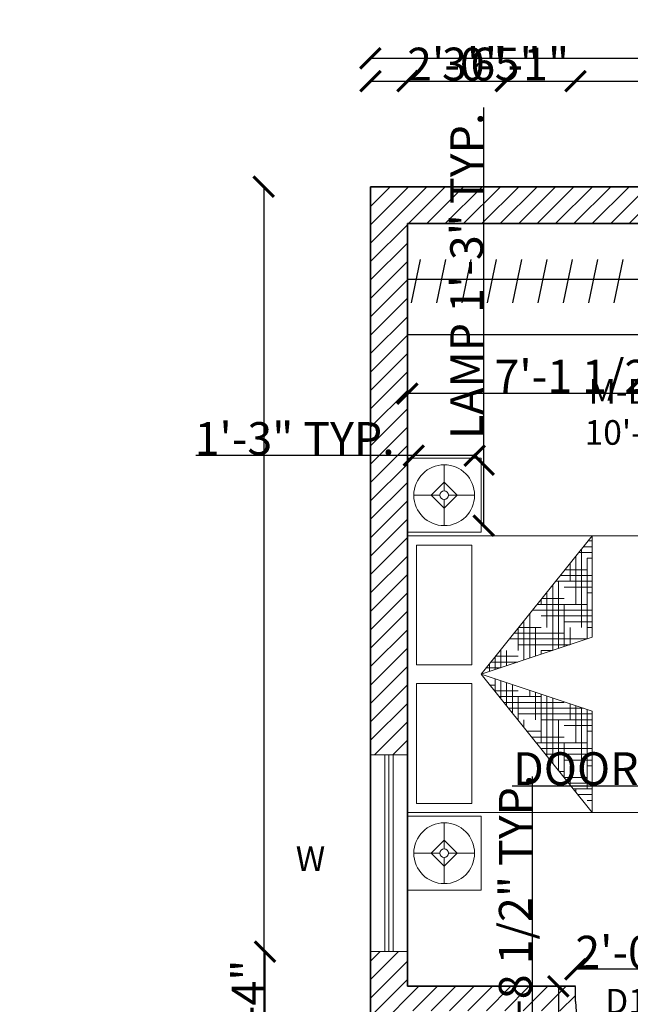
# Model space of a CAD drawing. Units: inches. Extents: x 2094 to 2639, y 1426 to 1997.
# Tile 5 of 8: x 2094 to 2243, y 1730 to 1970. Entities that reach past the tile are written whole.
import ezdxf

# ---------------------------------------------------------------- set-up
doc = ezdxf.new("R2010")
doc.units = ezdxf.units.IN
for name, color, linetype, lineweight in [('A-ANNO-DIMS', 2, 'Continuous', 18), ('A-ANNO-TEXT', 7, 'Continuous', 18), ('A-AREA-IDEN', 7, 'Continuous', 25), ('A-FLOR-CASE', 8, 'Continuous', 25), ('A-FURN', 8, 'Continuous', 18), ('A-WALL-PATT', 8, 'Continuous', 13), ('Doors', 34, 'Continuous', 25), ('Walls', 7, 'Continuous', 35), ('Windows', 150, 'Continuous', 18)]:
    doc.layers.add(name, color=color, linetype=linetype, lineweight=lineweight)
doc.styles.get("Standard").update_dxf_attribs({"font": 'arial.ttf'})
doc.dimstyles.get("Standard").update_dxf_attribs({"dimtxt": 8, "dimasz": 5, "dimexe": 0.18, "dimexo": 0.0625, "dimgap": 0.09, "dimtad": 1, "dimdec": 1, "dimzin": 0, "dimdsep": 46, "dimlunit": 4, "dimtxsty": 'Standard', "dimblk": 'ARCHTICK', "dimcen": 0.09, "dimse1": 1, "dimse2": 1, "dimadec": 0, "dimazin": 0, "dimtfac": 1, "dimtdec": 1, "dimtofl": 0, "dimtmove": 0, "dimatfit": 3, "dimfxl": 1, "dimtolj": 1, "dimtzin": 0, "dimarcsym": 0})

# ---------------------------------------------------------------- blocks, each defined once
blk = doc.blocks.new('*X3')
at = {"color": 0}
for p, q in [((20.199, 14.7812), (20.2772, 14.7812)), ((20.25, 14.8125), (20.2772, 14.8125)), ((20.1562, 14.625), (20.1562, 14.7281)), ((20.1739, 14.75), (20.2772, 14.75)), ((20.1875, 14.75), (20.1875, 14.7669)), ((20.25, 14.3194), (20.25, 14.75)), ((20.1236, 14.6875), (20.25, 14.6875)), ((20.125, 14.5), (20.125, 14.6893)), ((20.1487, 14.7188), (20.2772, 14.7188)), ((20.0938, 14.375), (20.0938, 14.6504)), ((20.0984, 14.6562), (20.125, 14.6562)), ((20.2188, 14.3091), (20.2188, 14.625)), ((20.25, 14.625), (20.2772, 14.625)), ((20.0312, 14.2469), (20.0312, 14.5727)), ((20.0625, 14.2573), (20.0625, 14.6116)), ((20.125, 14.5938), (20.2772, 14.5938)), ((19.9979, 14.5312), (20.2772, 14.5312)), ((20.023, 14.5625), (20.2772, 14.5625)), ((19.9476, 14.4688), (20.125, 14.4688)), ((19.9727, 14.5), (20.25, 14.5)), ((20, 14.2366), (20, 14.5)), ((20.1875, 14.2987), (20.1875, 14.5)), ((19.9062, 14.375), (19.9062, 14.4174)), ((19.9225, 14.4375), (20, 14.4375)), ((20.25, 14.4375), (20.2772, 14.4375)), ((19.875, 14.25), (19.875, 14.3785)), ((19.9688, 14.2262), (19.9688, 14.375)), ((20, 14.375), (20.2772, 14.375)), ((20.125, 14.4062), (20.2772, 14.4062)), ((20.1562, 14.2884), (20.1562, 14.375)), ((19.8125, 14.1744), (19.8125, 14.3008)), ((19.8219, 14.3125), (20.2291, 14.3125)), ((19.8438, 14.1848), (19.8438, 14.3397)), ((19.875, 14.3438), (20.2772, 14.3438)), ((19.7716, 14.25), (20, 14.25)), ((19.7812, 14.1641), (19.7812, 14.262)), ((19.7967, 14.2812), (20.125, 14.2812)), ((19.9375, 14.2159), (19.9375, 14.25)), ((19.7465, 14.2188), (19.875, 14.2188)), ((19.75, 14.1537), (19.75, 14.2231)), ((19.7213, 14.1875), (19.75, 14.1875)), ((19.7018, 14.0938), (19.7786, 14.0938)), ((19.7188, 14.0726), (19.7188, 14.1136)), ((19.75, 14.0338), (19.75, 14.1032)), ((19.7812, 13.9949), (19.7812, 14.0929)), ((19.7269, 14.0625), (19.8728, 14.0625)), ((19.8125, 14), (19.8125, 14.0825)), ((19.9062, 13.8396), (19.9062, 14.0514)), ((19.9375, 13.8007), (19.9375, 14.0411)), ((19.752, 14.0312), (19.875, 14.0312)), ((19.875, 13.8784), (19.875, 14)), ((19.9688, 13.875), (19.9688, 14.0307)), ((20, 14), (20, 14.0204)), ((20, 14), (20.0614, 14)), ((20.0625, 13.6454), (20.0625, 13.9996)), ((20.0938, 13.625), (20.0938, 13.9893)), ((19.8275, 13.9375), (20.25, 13.9375)), ((19.875, 13.9688), (20.1557, 13.9688)), ((20.125, 13.75), (20.125, 13.9789)), ((20.1562, 13.875), (20.1562, 13.9686)), ((20.25, 13.5), (20.25, 13.9375)), ((19.8526, 13.9062), (20.125, 13.9062)), ((19.8777, 13.875), (20, 13.875)), ((20.0312, 13.6842), (20.0312, 13.875)), ((20.2188, 13.4511), (20.2188, 13.875)), ((20.25, 13.875), (20.2772, 13.875)), ((20.125, 13.8438), (20.2772, 13.8438)), ((19.9532, 13.7812), (20.2772, 13.7812)), ((20, 13.8125), (20.2772, 13.8125)), ((19.9783, 13.75), (20.25, 13.75)), ((20, 13.723), (20, 13.75)), ((20.0035, 13.7188), (20.125, 13.7188)), ((20.1875, 13.49), (20.1875, 13.75)), ((20.25, 13.6875), (20.2772, 13.6875)), ((20.0789, 13.625), (20.2772, 13.625)), ((20.125, 13.6562), (20.2772, 13.6562)), ((20.1562, 13.5288), (20.1562, 13.625)), ((20.104, 13.5938), (20.2772, 13.5938)), ((20.1292, 13.5625), (20.25, 13.5625)), ((20.25, 13.5), (20.2772, 13.5)), ((20.2046, 13.4688), (20.2772, 13.4688)), ((20.2297, 13.4375), (20.2772, 13.4375)), ((20.2549, 13.4062), (20.2772, 13.4062))]:
    blk.add_line(p, q, dxfattribs=at)
blk = doc.blocks.new('MAT-P13')
for p, q in [((-1.17, 0), (-1.17, -0.4)), ((-1.17, 0), (-0.77, 0)), ((-0.77, 0), (-0.77, -0.4)), ((-0.75, 0), (0.75, 0)), ((-0.75, 0), (-0.75, -1.9)), ((0.75, 0), (0.75, -1.9)), ((0.77, 0), (1.17, 0)), ((0.77, 0), (0.77, -0.4)), ((1.17, 0), (1.17, -0.4)), ((-0.7, -0.05), (-0.7, -0.35)), ((-0.7, -0.05), (-0.05, -0.05)), ((-0.05, -0.35), (-0.05, -0.05)), ((0.05, -0.05), (0.7, -0.05)), ((0.05, -0.35), (0.05, -0.05)), ((0.7, -0.05), (0.7, -0.35)), ((-0.7, -0.35), (-0.05, -0.35)), ((0.05, -0.35), (0.7, -0.35)), ((-1.17, -0.4), (-0.77, -0.4)), ((-0.75, -1.0034), (0, -0.4)), ((0, -0.4), (-0.75, -1.0034)), ((0, -0.4), (-0.2, -1.0034)), ((0, -0.4), (0.2, -1.0034)), ((0, -0.4), (0.75, -1.0034)), ((0.77, -0.4), (1.17, -0.4)), ((-0.75, -1.0034), (-0.2, -1.0034)), ((0.2, -1.0034), (0.75, -1.0034)), ((0.75, -1.9), (-0.75, -1.9))]:
    blk.add_line(p, q)
at = {"xscale": -1, "rotation": 90}
blk.add_blockref('*X3', (14.1285, 19.2738), dxfattribs=at)
blk = doc.blocks.new('Lamp - Table')
for p, q in [((0, 7), (0, 1)), ((0, 3), (-3, 0)), ((3, 0), (0, 3)), ((-1, 0), (-7, 0)), ((-3, 0), (0, -3)), ((0, -3), (3, 0)), ((1, 0), (7, 0)), ((0, -1), (0, -7))]:
    blk.add_line(p, q)
for radius in [7, 1]:
    blk.add_circle((0, 0), radius)
blk = doc.blocks.new('AP0B05')
for p, q in [((35, 100), (35, 880)), ((75, 100), (75, 878.9)), ((35, 100), (35, -20)), ((815, 100), (815, -20))]:
    blk.add_line(p, q)
blk.add_lwpolyline([(35, 100), (75, 100)])
blk.add_arc((-2.4, 62.6), 818.3, 2.62122, 87.37878)
blk = doc.blocks.new('_ArchTick')
at = {"color": 0, "linetype": 'ByBlock', "const_width": 0.15}
blk.add_lwpolyline([(-0.5, -0.5), (0.5, 0.5)], dxfattribs=at)
blk = doc.blocks.new('*D13')
at = {"layer": 'A-ANNO-DIMS', "color": 0, "lineweight": -2, "transparency": 16777216}
blk.add_line((2180.06, 1960.22), (2537.06, 1960.22), dxfattribs=at)
at = {"layer": 'Defpoints', "color": 0, "transparency": 16777216}
for p in [(2537.06, 1960.22), (2180.06, 1928.9), (2537.06, 1928.9)]:
    blk.add_point(p, dxfattribs=at)
at = {"layer": 'A-ANNO-DIMS', "color": 0, "lineweight": -2, "transparency": 16777216, "xscale": 5, "yscale": 5, "zscale": 5, "rotation": 180}
blk.add_blockref('_ArchTick', (2180.06, 1960.22), dxfattribs=at)
at = {"layer": 'A-ANNO-DIMS', "color": 0, "lineweight": -2, "transparency": 16777216, "xscale": 5, "yscale": 5, "zscale": 5}
blk.add_blockref('_ArchTick', (2537.06, 1960.22), dxfattribs=at)
at = {"layer": 'A-ANNO-DIMS', "color": 0, "transparency": 16777216, "insert": (2358.56, 1964.39), "char_height": 8, "attachment_point": 5}
blk.add_mtext('\\A1;29\'-9"', dxfattribs=at)
blk = doc.blocks.new('*D14')
at = {"layer": 'A-ANNO-DIMS', "color": 0, "lineweight": -2, "transparency": 16777216}
blk.add_line((2154, 1928.9), (2154, 1459.9), dxfattribs=at)
at = {"layer": 'Defpoints', "color": 0, "transparency": 16777216}
for p in [(2180.06, 1928.9), (2154, 1459.9), (2180.06, 1459.9)]:
    blk.add_point(p, dxfattribs=at)
at = {"layer": 'A-ANNO-DIMS', "color": 0, "lineweight": -2, "transparency": 16777216, "xscale": 5, "yscale": 5, "zscale": 5}
for p, rotation in [((2154, 1928.9), 90), ((2154, 1459.9), 270)]:
    blk.add_blockref('_ArchTick', p, dxfattribs=dict(at, rotation=rotation))
at = {"layer": 'A-ANNO-DIMS', "color": 0, "transparency": 16777216, "insert": (2149.82, 1694.4), "char_height": 8, "attachment_point": 5, "rotation": 90}
blk.add_mtext('\\A1;39\'-1"', dxfattribs=at)
blk = doc.blocks.new('WIN-48IN')
for p, q in [((0, 5.5), (48, 5.5)), ((0, 4.5), (48, 4.5)), ((0, 3.5), (48, 3.5))]:
    blk.add_line(p, q)
blk.add_lwpolyline([(0, 0), (48, 0), (48, 9), (0, 9)], close=True)
blk = doc.blocks.new('*D23')
at = {"layer": 'A-ANNO-DIMS', "color": 0, "lineweight": -2, "transparency": 16777216}
for p, q in [((2225.93, 1733.9), (2225.93, 1706.16)), ((2225.93, 1706.16), (2225.93, 1624.84))]:
    blk.add_line(p, q, dxfattribs=at)
at = {"layer": 'Defpoints', "color": 0, "transparency": 16777216}
for p in [(2230.09, 1733.9), (2225.93, 1706.16), (2230.09, 1706.16)]:
    blk.add_point(p, dxfattribs=at)
at = {"layer": 'A-ANNO-DIMS', "color": 0, "lineweight": -2, "transparency": 16777216, "xscale": 5, "yscale": 5, "zscale": 5}
for p, rotation in [((2225.93, 1733.9), 90), ((2225.93, 1706.16), 270)]:
    blk.add_blockref('_ArchTick', p, dxfattribs=dict(at, rotation=rotation))
at = {"layer": 'A-ANNO-DIMS', "color": 0, "transparency": 16777216, "insert": (2221.69, 1663), "char_height": 8, "attachment_point": 5, "rotation": 90}
blk.add_mtext('\\A1;DOOR 2\'-3 1/2"', dxfattribs=at)
blk = doc.blocks.new('*D24')
at = {"layer": 'A-ANNO-DIMS', "color": 0, "lineweight": -2, "transparency": 16777216}
blk.add_line((2254.12, 1738.06), (2230.09, 1738.06), dxfattribs=at)
at = {"layer": 'Defpoints', "color": 0, "transparency": 16777216}
for p in [(2230.09, 1738.06), (2230.09, 1733.9), (2254.12, 1733.9)]:
    blk.add_point(p, dxfattribs=at)
at = {"layer": 'A-ANNO-DIMS', "color": 0, "lineweight": -2, "transparency": 16777216, "xscale": 5, "yscale": 5, "zscale": 5, "rotation": 180}
blk.add_blockref('_ArchTick', (2230.09, 1738.06), dxfattribs=at)
at = {"layer": 'A-ANNO-DIMS', "color": 0, "lineweight": -2, "transparency": 16777216, "xscale": 5, "yscale": 5, "zscale": 5}
blk.add_blockref('_ArchTick', (2254.12, 1738.06), dxfattribs=at)
at = {"layer": 'A-ANNO-DIMS', "color": 0, "transparency": 16777216, "insert": (2242.11, 1742.23), "char_height": 8, "attachment_point": 5}
blk.add_mtext('\\A1;2\'-0"', dxfattribs=at)
blk = doc.blocks.new('*D25')
at = {"layer": 'A-ANNO-DIMS', "color": 0, "lineweight": -2, "transparency": 16777216}
for p, q in [((2277.31, 1782.75), (2214.62, 1782.75)), ((2318.06, 1782.75), (2277.31, 1782.75))]:
    blk.add_line(p, q, dxfattribs=at)
at = {"layer": 'Defpoints', "color": 0, "transparency": 16777216}
for p in [(2277.31, 1782.75), (2277.31, 1776.64), (2318.06, 1776.64)]:
    blk.add_point(p, dxfattribs=at)
at = {"layer": 'A-ANNO-DIMS', "color": 0, "lineweight": -2, "transparency": 16777216, "xscale": 5, "yscale": 5, "zscale": 5, "rotation": 180}
blk.add_blockref('_ArchTick', (2277.31, 1782.75), dxfattribs=at)
at = {"layer": 'A-ANNO-DIMS', "color": 0, "lineweight": -2, "transparency": 16777216, "xscale": 5, "yscale": 5, "zscale": 5}
blk.add_blockref('_ArchTick', (2318.06, 1782.75), dxfattribs=at)
at = {"layer": 'A-ANNO-DIMS', "color": 0, "transparency": 16777216, "insert": (2243.46, 1786.98), "char_height": 8, "attachment_point": 5}
blk.add_mtext('\\A1;DOOR 3\'-5"', dxfattribs=at)
blk = doc.blocks.new('*D34')
at = {"layer": 'A-ANNO-DIMS', "color": 0, "lineweight": -2, "transparency": 16777216}
blk.add_line((2274.56, 1878.47), (2189.06, 1878.47), dxfattribs=at)
at = {"layer": 'Defpoints', "color": 0, "transparency": 16777216}
for p in [(2189.06, 1878.47), (2189.06, 1862.67), (2274.56, 1862.67)]:
    blk.add_point(p, dxfattribs=at)
at = {"layer": 'A-ANNO-DIMS', "color": 0, "lineweight": -2, "transparency": 16777216, "xscale": 5, "yscale": 5, "zscale": 5, "rotation": 180}
blk.add_blockref('_ArchTick', (2189.06, 1878.47), dxfattribs=at)
at = {"layer": 'A-ANNO-DIMS', "color": 0, "lineweight": -2, "transparency": 16777216, "xscale": 5, "yscale": 5, "zscale": 5}
blk.add_blockref('_ArchTick', (2274.56, 1878.47), dxfattribs=at)
at = {"layer": 'A-ANNO-DIMS', "color": 0, "transparency": 16777216, "insert": (2231.81, 1882.7), "char_height": 8, "attachment_point": 5}
blk.add_mtext('\\A1;7\'-1 1/2"', dxfattribs=at)
blk = doc.blocks.new('*D37')
at = {"layer": 'A-ANNO-DIMS', "color": 0, "lineweight": -2, "transparency": 16777216}
for p, q in [((2207.7, 1861.1), (2207.7, 1948.22)), ((2207.7, 1846.25), (2207.7, 1861.1))]:
    blk.add_line(p, q, dxfattribs=at)
at = {"layer": 'Defpoints', "color": 0, "transparency": 16777216}
for p in [(2205.48, 1861.1), (2207.7, 1861.1), (2205.48, 1846.25)]:
    blk.add_point(p, dxfattribs=at)
at = {"layer": 'A-ANNO-DIMS', "color": 0, "lineweight": -2, "transparency": 16777216, "xscale": 5, "yscale": 5, "zscale": 5}
for p, rotation in [((2207.7, 1861.1), 90), ((2207.7, 1846.25), 270)]:
    blk.add_blockref('_ArchTick', p, dxfattribs=dict(at, rotation=rotation))
at = {"layer": 'A-ANNO-DIMS', "color": 0, "transparency": 16777216, "insert": (2203.53, 1907.16), "char_height": 8, "attachment_point": 5, "rotation": 90}
blk.add_mtext('\\A1;LAMP 1\'-3" TYP.', dxfattribs=at)
blk = doc.blocks.new('*D38')
at = {"layer": 'A-ANNO-DIMS', "color": 0, "lineweight": -2, "transparency": 16777216}
for p, q in [((2190.64, 1863.32), (2137.44, 1863.32)), ((2205.48, 1863.32), (2190.64, 1863.32))]:
    blk.add_line(p, q, dxfattribs=at)
at = {"layer": 'Defpoints', "color": 0, "transparency": 16777216}
for p in [(2190.64, 1863.32), (2190.64, 1861.1), (2205.48, 1861.1)]:
    blk.add_point(p, dxfattribs=at)
at = {"layer": 'A-ANNO-DIMS', "color": 0, "lineweight": -2, "transparency": 16777216, "xscale": 5, "yscale": 5, "zscale": 5, "rotation": 180}
blk.add_blockref('_ArchTick', (2190.64, 1863.32), dxfattribs=at)
at = {"layer": 'A-ANNO-DIMS', "color": 0, "lineweight": -2, "transparency": 16777216, "xscale": 5, "yscale": 5, "zscale": 5}
blk.add_blockref('_ArchTick', (2205.48, 1863.32), dxfattribs=at)
at = {"layer": 'A-ANNO-DIMS', "color": 0, "transparency": 16777216, "insert": (2161.54, 1867.5), "char_height": 8, "attachment_point": 5}
blk.add_mtext('\\A1;1\'-3" TYP.', dxfattribs=at)
blk = doc.blocks.new('*D39')
at = {"layer": 'A-ANNO-DIMS', "color": 0, "lineweight": -2, "transparency": 16777216}
for p, q in [((2189.06, 1717.27), (2094.42, 1717.27)), ((2215.64, 1717.27), (2189.06, 1717.27))]:
    blk.add_line(p, q, dxfattribs=at)
at = {"layer": 'Defpoints', "color": 0, "transparency": 16777216}
for p in [(2189.06, 1717.27), (2189.06, 1713.28), (2215.64, 1713.28)]:
    blk.add_point(p, dxfattribs=at)
at = {"layer": 'A-ANNO-DIMS', "color": 0, "lineweight": -2, "transparency": 16777216, "xscale": 5, "yscale": 5, "zscale": 5, "rotation": 180}
blk.add_blockref('_ArchTick', (2189.06, 1717.27), dxfattribs=at)
at = {"layer": 'A-ANNO-DIMS', "color": 0, "lineweight": -2, "transparency": 16777216, "xscale": 5, "yscale": 5, "zscale": 5}
blk.add_blockref('_ArchTick', (2215.64, 1717.27), dxfattribs=at)
at = {"layer": 'A-ANNO-DIMS', "color": 0, "transparency": 16777216, "insert": (2139.24, 1721.49), "char_height": 8, "attachment_point": 5}
blk.add_mtext('\\A1;WC 2\'-2 1/2" TYP.', dxfattribs=at)
blk = doc.blocks.new('*D40')
at = {"layer": 'A-ANNO-DIMS', "color": 0, "lineweight": -2, "transparency": 16777216}
for p, q in [((2219.63, 1713.28), (2219.63, 1785.11)), ((2219.63, 1692.99), (2219.63, 1713.28))]:
    blk.add_line(p, q, dxfattribs=at)
at = {"layer": 'Defpoints', "color": 0, "transparency": 16777216}
for p in [(2215.64, 1713.28), (2219.63, 1713.28), (2215.64, 1692.99)]:
    blk.add_point(p, dxfattribs=at)
at = {"layer": 'A-ANNO-DIMS', "color": 0, "lineweight": -2, "transparency": 16777216, "xscale": 5, "yscale": 5, "zscale": 5}
for p, rotation in [((2219.63, 1713.28), 90), ((2219.63, 1692.99), 270)]:
    blk.add_blockref('_ArchTick', p, dxfattribs=dict(at, rotation=rotation))
at = {"layer": 'A-ANNO-DIMS', "color": 0, "transparency": 16777216, "insert": (2215.41, 1751.7), "char_height": 8, "attachment_point": 5, "rotation": 90}
blk.add_mtext('\\A1;1\'-8 1/2" TYP.', dxfattribs=at)
blk = doc.blocks.new('*D53')
at = {"layer": 'A-ANNO-DIMS', "color": 0, "lineweight": -2, "transparency": 16777216}
blk.add_line((2180.06, 1954.65), (2252.94, 1954.65), dxfattribs=at)
at = {"layer": 'Defpoints', "color": 0, "transparency": 16777216}
for p in [(2252.94, 1954.65), (2180.06, 1928.9), (2252.94, 1928.9)]:
    blk.add_point(p, dxfattribs=at)
at = {"layer": 'A-ANNO-DIMS', "color": 0, "lineweight": -2, "transparency": 16777216, "xscale": 5, "yscale": 5, "zscale": 5, "rotation": 180}
blk.add_blockref('_ArchTick', (2180.06, 1954.65), dxfattribs=at)
at = {"layer": 'A-ANNO-DIMS', "color": 0, "lineweight": -2, "transparency": 16777216, "xscale": 5, "yscale": 5, "zscale": 5}
blk.add_blockref('_ArchTick', (2252.94, 1954.65), dxfattribs=at)
at = {"layer": 'A-ANNO-DIMS', "color": 0, "transparency": 16777216, "insert": (2216.5, 1958.82), "char_height": 8, "attachment_point": 5}
blk.add_mtext('\\A1;6\'-1"', dxfattribs=at)
blk = doc.blocks.new('*D58')
at = {"layer": 'A-ANNO-DIMS', "color": 0, "lineweight": -2, "transparency": 16777216}
blk.add_line((2154.31, 1714.4), (2154.31, 1742.37), dxfattribs=at)
at = {"layer": 'Defpoints', "color": 0, "transparency": 16777216}
for p in [(2154.31, 1742.37), (2180.06, 1742.37), (2180.06, 1714.4)]:
    blk.add_point(p, dxfattribs=at)
at = {"layer": 'A-ANNO-DIMS', "color": 0, "lineweight": -2, "transparency": 16777216, "xscale": 5, "yscale": 5, "zscale": 5}
for p, rotation in [((2154.31, 1742.37), 90), ((2154.31, 1714.4), 270)]:
    blk.add_blockref('_ArchTick', p, dxfattribs=dict(at, rotation=rotation))
at = {"layer": 'A-ANNO-DIMS', "color": 0, "transparency": 16777216, "insert": (2150.2, 1728.38), "char_height": 8, "attachment_point": 5, "rotation": 90}
blk.add_mtext('\\A1;2\'-4"', dxfattribs=at)
blk = doc.blocks.new('*D68')
at = {"layer": 'A-ANNO-DIMS', "color": 0, "lineweight": -2, "transparency": 16777216}
blk.add_line((2189.06, 1954.65), (2213.06, 1954.65), dxfattribs=at)
at = {"layer": 'Defpoints', "color": 0, "transparency": 16777216}
for p in [(2213.06, 1954.65), (2189.06, 1670.9), (2213.06, 1670.9)]:
    blk.add_point(p, dxfattribs=at)
at = {"layer": 'A-ANNO-DIMS', "color": 0, "lineweight": -2, "transparency": 16777216, "xscale": 5, "yscale": 5, "zscale": 5, "rotation": 180}
blk.add_blockref('_ArchTick', (2189.06, 1954.65), dxfattribs=at)
at = {"layer": 'A-ANNO-DIMS', "color": 0, "lineweight": -2, "transparency": 16777216, "xscale": 5, "yscale": 5, "zscale": 5}
blk.add_blockref('_ArchTick', (2213.06, 1954.65), dxfattribs=at)
at = {"layer": 'A-ANNO-DIMS', "color": 0, "transparency": 16777216, "insert": (2201.06, 1958.82), "char_height": 8, "attachment_point": 5}
blk.add_mtext('\\A1;2\'-0"', dxfattribs=at)
blk = doc.blocks.new('*D70')
at = {"layer": 'A-ANNO-DIMS', "color": 0, "lineweight": -2, "transparency": 16777216}
blk.add_line((2189.06, 1954.65), (2230.09, 1954.65), dxfattribs=at)
at = {"layer": 'Defpoints', "color": 0, "transparency": 16777216}
for p in [(2230.09, 1954.65), (2189.06, 1733.9), (2230.09, 1733.9)]:
    blk.add_point(p, dxfattribs=at)
at = {"layer": 'A-ANNO-DIMS', "color": 0, "lineweight": -2, "transparency": 16777216, "xscale": 5, "yscale": 5, "zscale": 5, "rotation": 180}
blk.add_blockref('_ArchTick', (2189.06, 1954.65), dxfattribs=at)
at = {"layer": 'A-ANNO-DIMS', "color": 0, "lineweight": -2, "transparency": 16777216, "xscale": 5, "yscale": 5, "zscale": 5}
blk.add_blockref('_ArchTick', (2230.09, 1954.65), dxfattribs=at)
at = {"layer": 'A-ANNO-DIMS', "color": 0, "transparency": 16777216, "insert": (2209.57, 1958.83), "char_height": 8, "attachment_point": 5}
blk.add_mtext('\\A1;3\'-5"', dxfattribs=at)

msp = doc.modelspace()

# ---------------------------------------------------------------- hatches: boundary and pattern name
at = {"layer": 'A-WALL-PATT', "transparency": 33554585}
h = msp.add_hatch(dxfattribs=at)
h.set_pattern_fill('ANSI31', color=256)
h.paths.add_polyline_path([(2189.06, 1727.9), (2230.3, 1727.9, -0.022928), (2230.09, 1730.2), (2230.09, 1733.9), (2189.06, 1733.9), (2189.06, 1742.37), (2180.06, 1742.37), (2180.06, 1714.4), (2189.06, 1714.4)])
h.paths.add_polyline_path([(2456.51, 1574.9), (2413.83, 1574.9), (2413.83, 1565.9), (2456.51, 1565.9)])
h.paths.add_polyline_path([(2537.06, 1643.81), (2528.06, 1643.81), (2528.06, 1574.9), (2519.78, 1574.9), (2519.78, 1571.88), (2519.78, 1565.9), (2537.06, 1565.9)])
h.paths.add_polyline_path([(2339.06, 1928.9), (2300.94, 1928.9), (2300.94, 1919.9), (2309.06, 1919.9), (2309.06, 1776.3, -0.024186), (2312.62, 1776.64), (2318.06, 1776.64), (2318.06, 1778.9), (2336.06, 1778.9), (2336.06, 1787.9), (2318.06, 1787.9), (2318.06, 1835.9), (2384.06, 1835.9), (2384.06, 1787.9), (2366.06, 1787.9), (2366.06, 1778.9), (2479.64, 1778.9), (2479.64, 1784.88, -0.018603), (2479.89, 1787.9), (2390.06, 1787.9), (2390.06, 1847.57), (2385.61, 1847.57), (2384.06, 1847.57), (2384.06, 1841.9), (2318.06, 1841.9), (2318.06, 1919.9), (2339.06, 1919.9)])
h.paths.add_polyline_path([(2252.94, 1928.9), (2180.06, 1928.9), (2180.06, 1790.37), (2189.06, 1790.37), (2189.06, 1843.77), (2189.06, 1919.9), (2252.94, 1919.9)])
h.paths.add_polyline_path([(2472.33, 1928.9), (2363.06, 1928.9), (2363.06, 1919.9), (2384.06, 1919.9), (2384.06, 1876.38, -0.012802), (2385.61, 1876.49), (2390.06, 1876.49), (2390.06, 1919.9), (2472.33, 1919.9)], flags=17)
h.paths.add_polyline_path([(2537.06, 1928.9), (2520.33, 1928.9), (2520.33, 1919.9), (2528.06, 1919.9), (2528.06, 1905.95), (2528.06, 1787.9), (2518.5, 1787.9), (2518.5, 1784.88), (2518.5, 1778.9), (2528.06, 1778.9), (2528.06, 1715.81), (2537.06, 1715.81)])
h.paths.add_polyline_path([(2379.33, 1857.12), (2393.06, 1857.12), (2393.06, 1866.16), (2379.33, 1866.16)], flags=25)
h.paths.add_polyline_path([(2235.85, 1725.77), (2249.57, 1725.77), (2249.57, 1734.81), (2235.85, 1734.81)], flags=25)
h.paths.add_polyline_path([(2305.79, 1754.6), (2314.84, 1754.6), (2314.84, 1763.6), (2305.79, 1763.6)], flags=9)
h.paths.add_polyline_path([(2493.85, 1778.22), (2502.9, 1778.22), (2502.9, 1787.22), (2493.85, 1787.22)], flags=9)
h.paths.add_polyline_path([(2370.69, 1555.65), (2381.6, 1555.65), (2381.6, 1564.65), (2370.69, 1564.65)], flags=9)
h.paths.add_polyline_path([(2461.57, 1555.65), (2477.6, 1555.65), (2477.6, 1564.65), (2461.57, 1564.65)], flags=9)
h.paths.add_polyline_path([(2493.18, 1565.15), (2509.22, 1565.15), (2509.22, 1574.15), (2493.18, 1574.15)], flags=9)
h.paths.add_polyline_path([(2408.32, 1501.7), (2449.12, 1501.7), (2449.12, 1520.36), (2408.32, 1520.36)], flags=9)
h.paths.add_polyline_path([(2398.49, 1698.6), (2441.61, 1698.6), (2441.61, 1717.26), (2398.49, 1717.26)], flags=9)
h.paths.add_polyline_path([(2248.63, 1683.29), (2287.87, 1683.29), (2287.87, 1701.95), (2248.63, 1701.95)], flags=25)
h.paths.add_polyline_path([(2440.73, 1823.2), (2483.86, 1823.2), (2483.86, 1841.85), (2440.73, 1841.85)], flags=9)
h.paths.add_polyline_path([(2335.3, 1804.5), (2370.65, 1804.5), (2370.65, 1823.15), (2335.3, 1823.15)], flags=25)
h.paths.add_polyline_path([(2335.3, 1893.12), (2370.65, 1893.12), (2370.65, 1911.77), (2335.3, 1911.77)], flags=25)
h.paths.add_polyline_path([(2241.82, 1863.6), (2290.11, 1863.6), (2290.11, 1882.25), (2241.82, 1882.25)], flags=9)

# ---------------------------------------------------------------- linework, layer by layer
at = {"layer": 'A-FLOR-CASE'}
for p, q in [((2192.2, 1911.13), (2190, 1900.57)), ((2198.38, 1911.13), (2196.18, 1900.57)), ((2204.57, 1911.13), (2202.37, 1900.57)), ((2210.76, 1911.13), (2208.56, 1900.57)), ((2216.95, 1911.13), (2214.75, 1900.57)), ((2223.13, 1911.13), (2220.93, 1900.57)), ((2229.32, 1911.13), (2227.12, 1900.57)), ((2235.51, 1911.13), (2233.31, 1900.57)), ((2241.7, 1911.13), (2239.5, 1900.57)), ((2189.06, 1906.33), (2252.26, 1906.33))]:
    msp.add_line(p, q, dxfattribs=at)
msp.add_lwpolyline([(2189.06, 1919.9), (2252.26, 1919.9), (2252.26, 1892.76), (2189.06, 1892.76)], close=True, dxfattribs=at)
at = {"layer": 'Walls'}
for p, q in [((2180.06, 1928.9), (2537.06, 1928.9)), ((2180.06, 1928.9), (2180.06, 1459.9)), ((2189.06, 1919.9), (2309.06, 1919.9)), ((2189.06, 1919.9), (2189.06, 1733.9)), ((2189.06, 1733.9), (2230.09, 1733.9))]:
    msp.add_line(p, q, dxfattribs=at)

# ---------------------------------------------------------------- block references
at = {"layer": 'A-FURN', "rotation": 90}
for name, p, xscale, yscale, zscale in [('MAT-P13', (2189.06, 1810.02), 45.00172282535224, 45.00172282535224, 45.00172282535224), ('Lamp - Table', (2198.06, 1853.67), 1.060186597105617, 1.060186597105617, 1.060186597105617), ('Lamp - Table', (2198.06, 1766.37), 1.060186597105617, 1.060186597105617, 1.060186597105617)]:
    msp.add_blockref(name, p, dxfattribs=dict(at, xscale=xscale, yscale=yscale, zscale=zscale))
at = {"layer": 'Doors', "xscale": 0.0308176600246466, "yscale": 0.0308176600246466, "zscale": 0.0308176600246466, "rotation": 180}
msp.add_blockref('AP0B05', (2255.2, 1733.28), dxfattribs=at)
at = {"layer": 'Windows', "rotation": 89.99999999999953}
msp.add_blockref('WIN-48IN', (2189.06, 1742.37), dxfattribs=at)

# ---------------------------------------------------------------- texts
at = {"layer": 'A-ANNO-TEXT'}
for s, p in [('W', (2161.82, 1762.02)), ('D1', (2237.35, 1727.28))]:
    msp.add_text(s, height=6, dxfattribs=at).set_placement(p)
at = {"layer": 'A-AREA-IDEN', "insert": (2231.43, 1881.98), "char_height": 6, "attachment_point": 1}
msp.add_mtext_dynamic_manual_height_columns("\\pxqc;M-BEDROOM\\P10'-0''X15'-6''", width=53.0999, gutter_width=63.55, heights=[0], dxfattribs=at)

# ---------------------------------------------------------------- dimensions: what is measured, and where the dimension line sits
at = {"layer": 'A-ANNO-DIMS'}
for base, p1, p2, override, picture, middle in [((2537.06, 1960.22), (2180.06, 1928.9), (2537.06, 1928.9), {"dimclrd": 0, "dimclre": 0, "dimclrt": 0}, '*D13', (2358.56, 1964.39)), ((2252.94, 1954.65), (2180.06, 1928.9), (2252.94, 1928.9), {"dimdec": 1, "dimlfac": 1, "dimrnd": 0, "dimzin": 1, "dimdsep": 46, "dimlunit": 4, "dimfrac": 2}, '*D53', (2216.5, 1958.82)), ((2230.09, 1954.65), (2189.06, 1733.9), (2230.09, 1733.9), {"dimdec": 1, "dimlfac": 1, "dimrnd": 0, "dimzin": 1, "dimdsep": 46, "dimlunit": 4, "dimfrac": 2}, '*D70', (2209.57, 1958.83)), ((2213.06, 1954.65), (2189.06, 1670.9), (2213.06, 1670.9), {"dimdec": 1, "dimlfac": 1, "dimrnd": 0, "dimzin": 1, "dimdsep": 46, "dimlunit": 4, "dimfrac": 2}, '*D68', (2201.06, 1958.82))]:
    dim = msp.add_linear_dim(base=base, p1=p1, p2=p2, dimstyle='Standard', override=override, dxfattribs=at)
    dim.commit()
    dim.dimension.update_dxf_attribs({"geometry": picture, "text_midpoint": middle})
for base, p1, p2, angle, text, picture, middle in [((2207.7044, 1861.0959), (2205.478, 1846.2532), (2205.478, 1861.0959), 90, 'LAMP <> TYP.', '*D37', (2203.527, 1907.1599)), ((2190.64, 1863.32), (2205.48, 1861.1), (2190.64, 1861.1), 180, '<> TYP.', '*D38', (2161.54, 1867.5)), ((2277.3052, 1782.7522), (2318.0563, 1776.6396), (2277.3052, 1776.6396), 180, 'DOOR <>', '*D25', (2243.4648, 1786.9841)), ((2219.63, 1713.28), (2215.64, 1692.99), (2215.64, 1713.28), 90, '<> TYP.', '*D40', (2215.41, 1751.7)), ((2189.06, 1717.27), (2215.64, 1713.28), (2189.06, 1713.28), 180, 'WC <> TYP.', '*D39', (2139.24, 1721.49)), ((2225.93, 1706.16), (2230.09, 1733.9), (2230.09, 1706.16), 270, 'DOOR <>', '*D23', (2221.69, 1663))]:
    dim = msp.add_linear_dim(base=base, p1=p1, p2=p2, angle=angle, text=text, dimstyle='Standard', override={"dimdec": 1, "dimlfac": 1, "dimrnd": 0, "dimzin": 1, "dimdsep": 46, "dimlunit": 4, "dimfrac": 2}, dxfattribs=at)
    dim.commit()
    dim.dimension.update_dxf_attribs({"geometry": picture, "text_midpoint": middle})
for base, p1, p2, angle, override, picture, middle in [((2154, 1459.9), (2180.06, 1928.9), (2180.06, 1459.9), 90, {"dimclrd": 0, "dimclre": 0, "dimclrt": 0}, '*D14', (2149.82, 1694.4)), ((2189.06, 1878.47), (2274.56, 1862.67), (2189.06, 1862.67), 180, {"dimdec": 1, "dimlfac": 1, "dimrnd": 0, "dimzin": 1, "dimdsep": 46, "dimlunit": 4, "dimfrac": 2}, '*D34', (2231.81, 1882.7)), ((2230.09, 1738.06), (2254.12, 1733.9), (2230.09, 1733.9), 180, {"dimdec": 1, "dimlfac": 1, "dimrnd": 0, "dimzin": 1, "dimdsep": 46, "dimlunit": 4, "dimfrac": 2}, '*D24', (2242.11, 1742.23)), ((2154.31, 1742.37), (2180.06, 1714.4), (2180.06, 1742.37), 90, {"dimdec": 1, "dimlfac": 1, "dimrnd": 0, "dimzin": 1, "dimdsep": 46, "dimlunit": 4, "dimfrac": 2}, '*D58', (2150.2, 1728.38))]:
    dim = msp.add_linear_dim(base=base, p1=p1, p2=p2, angle=angle, dimstyle='Standard', override=override, dxfattribs=at)
    dim.commit()
    dim.dimension.update_dxf_attribs({"geometry": picture, "text_midpoint": middle})

doc.saveas('drawing.dxf')
